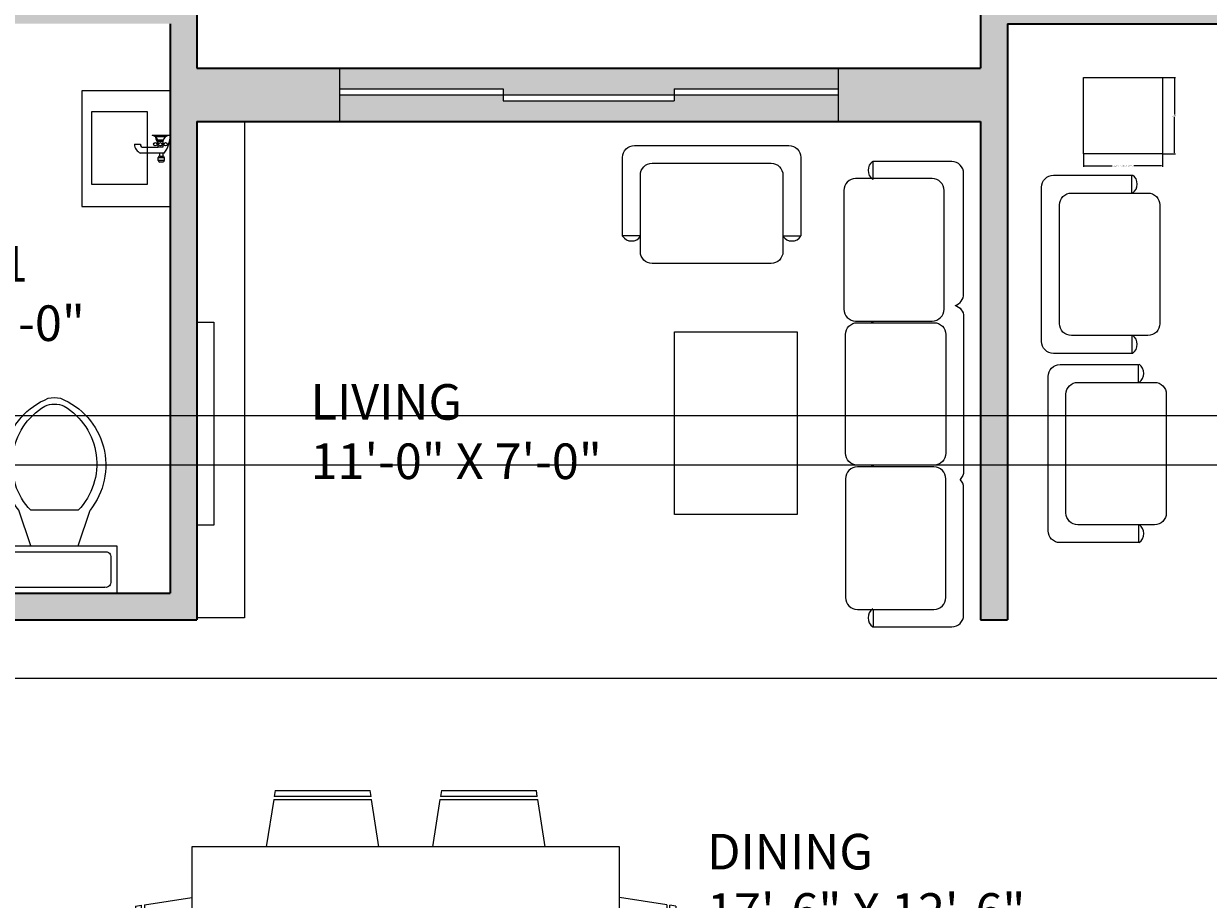
# Model space of a CAD drawing. Units: inches. Extents: x 1693 to 2974, y 2201 to 2965.
# Tile 12 of 24: x 1976 to 2175, y 2550 to 2698. Entities that reach past the tile are written whole.
import ezdxf

# ---------------------------------------------------------------- set-up
doc = ezdxf.new("R2010")
doc.units = ezdxf.units.IN
doc.header["$LTSCALE"] = 2
doc.header["$MEASUREMENT"] = 0
for name, color, linetype, lineweight in [('A-ANNO-DIMS', 2, 'Continuous', 18), ('A-AREA-IDEN', 7, 'Continuous', 18), ('A-DOOR', 3, 'Continuous', 25), ('A-FLOR-FIXT', 9, 'Continuous', 18), ('A-FURN', 8, 'Continuous', 18), ('A-WALL', 7, 'Continuous', 35)]:
    doc.layers.add(name, color=color, linetype=linetype, lineweight=lineweight)
doc.layers.add('A-GLAZ-PATT', color=141, linetype='Continuous', lineweight=13, true_color=0xadddf7)
doc.layers.add('A-WALL-PATT', color=251, linetype='Continuous', lineweight=13, true_color=0x636466)
doc.styles.get("Standard").update_dxf_attribs({"font": 'arial.ttf'})
doc.dimstyles.get("Standard").update_dxf_attribs({"dimtxt": 0.18, "dimasz": 0.18, "dimexe": 0.18, "dimexo": 0.0625, "dimgap": 0.09, "dimtad": 0, "dimtih": 1, "dimtoh": 1, "dimdec": 1, "dimzin": 0, "dimdsep": 46, "dimlunit": 3, "dimtxsty": 'Standard', "dimcen": 0.09, "dimadec": 0, "dimazin": 0, "dimtfac": 1, "dimtdec": 1, "dimtofl": 0, "dimtmove": 0, "dimatfit": 3, "dimfxl": 1, "dimtolj": 1, "dimtzin": 0, "dimarcsym": 0})

# ---------------------------------------------------------------- blocks, each defined once
blk = doc.blocks.new('Faucet - Bathroom side')
for p, q in [((-0.625, 4.25), (0.375, 4.25)), ((0.375, 3.75), (-0.625, 3.75)), ((-0.625, 3), (3.375, 3)), ((-0.375, 3), (-0.375, 3.5)), ((0.125, 3.5), (0.125, 3)), ((2.875, 2), (0.375, 2)), ((-1.625, 0), (-1.375, 0)), ((-1.375, 0), (1.375, 0)), ((-0.88366, 0.25), (0.88424, 0.25)), ((-0.375, 1.625), (-0.625, 1.625)), ((-0.375, 1.375), (-0.625, 1.375)), ((0.48078, 0.75), (-0.47286, 0.75)), ((0.375, 1.625), (0.625, 1.625)), ((0.375, 1.375), (0.625, 1.375)), ((4.375, 1.5), (3.375, 1.5))]:
    blk.add_line(p, q)
for points in [[(-0.625, 3.75), (-0.625, 4.25)], [(-0.375, 4.5), (0.125, 4.5)], [(0.375, 4.25), (0.375, 3.75)], [(0.125, 3.5), (-0.375, 3.5)]]:
    blk.add_lwpolyline(points)
blk.add_lwpolyline([(-0.375, 1), (-0.375, 2), (0.375, 2), (0.375, 1)], close=True)
for centre in [(-0.875, 1.5), (0, 1.5), (0.875, 1.5)]:
    blk.add_circle(centre, 0.27951)
for centre, radius, start, end in [((-0.38253, 4.2575), 0.24259, 88.22243, 181.7776), ((0.13252, 4.2575), 0.24259, 358.2224, 91.77757), ((3.45929, -0.0281), 5.08436, 143.4467, 179.6834), ((-0.38253, 3.7424), 0.24259, 178.2224, 271.7776), ((0.13252, 3.7424), 0.24259, 268.2224, 1.777565), ((2.96867, 1.5936), 0.41699, 347.0192, 102.9808), ((2.70708, 1.4714), 1.66816, 0.9827695, 66.39737), ((-1.75, 1.375), 1.42522, 285.2551, 344.7449), ((1.75, 1.375), 1.42522, 195.2551, 254.7449), ((-2.49562, -0.286), 3.38273, 9.709485, 29.48735)]:
    blk.add_arc(centre, radius, start, end)
blk = doc.blocks.new('Toilet - top')
for p, q in [((9.5, -6), (9.5, -2)), ((-10, -8.5), (-8, -8.5)), ((-10, -9.5), (-10, -8.5)), ((-7, -9.5), (-10, -9.5)), ((-8, -8.5), (-8, -8)), ((-7, -8), (-7, -9.5)), ((-4, -8), (-6, -14)), ((4, -8), (6, -14)), ((4, -14), (-4, -14))]:
    blk.add_line(p, q)
blk.add_lwpolyline([(10.5, -8), (10.5, 0), (-10.5, 0), (-10.5, -8)], close=True)
for points in [[(8.5, -1), (-8.5, -1)], [(-9.5, -2), (-9.5, -6)], [(-8.5, -7), (8.5, -7)]]:
    blk.add_lwpolyline(points)
for centre, radius, start, end in [((-8.62, -1.88), 0.884, 81.8699, 188.1301), ((8.62, -1.88), 0.884, 351.8699, 98.1301), ((-8.62, -6.12), 0.884, 171.8699, 278.1301), ((8.62, -6.12), 0.884, 261.8699, 8.1301), ((3.52, -21.58), 12.17, 141.4691, 247.9714), ((4.2, -21.82), 11.33, 136.3677, 238.9468), ((-3.52, -21.58), 12.17, 292.0284, 38.5307), ((-4.2, -21.82), 11.33, 301.053, 43.6321), ((0, -27.88), 4, 245.7318, 294.2682), ((0, -29), 4, 254.8605, 285.1395)]:
    blk.add_arc(centre, radius, start, end)
blk = doc.blocks.new('DINING-SET-72x36-6-SEAT')
for p, q in [((23.5, 55), (23.34, 54)), ((39.66, 54), (23.35, 54)), ((23.5, 55), (39.5, 55)), ((39.66, 54), (39.5, 55)), ((51.5, 55), (51.34, 54)), ((67.66, 54), (51.35, 54)), ((51.5, 55), (67.5, 55)), ((67.66, 54), (67.5, 55)), ((23.27, 53.5), (22.02, 45.5)), ((23.27, 53.5), (39.74, 53.5)), ((40.98, 45.5), (39.73, 53.5)), ((51.27, 53.5), (50.02, 45.5)), ((51.27, 53.5), (67.74, 53.5)), ((68.98, 45.5), (67.73, 53.5)), ((81.5, 45.5), (9.5, 45.5)), ((9.5, 45.5), (9.5, 9.5)), ((81.5, 9.5), (81.5, 45.5)), ((1.5, 35.73), (9.5, 36.98)), ((89.5, 35.73), (81.5, 36.98)), ((0, 35.5), (1, 35.66)), ((0, 35.5), (0, 19.5)), ((1, 19.34), (1, 35.65)), ((1.5, 35.73), (1.5, 19.26)), ((89.5, 35.73), (89.5, 19.26)), ((91, 35.5), (90, 35.66)), ((90, 19.34), (90, 35.65)), ((91, 35.5), (91, 19.5)), ((1, 19.34), (0, 19.5)), ((9.5, 18.02), (1.5, 19.27)), ((81.5, 18.02), (89.5, 19.27)), ((90, 19.34), (91, 19.5)), ((9.5, 9.5), (81.5, 9.5)), ((23.27, 1.5), (22.02, 9.5)), ((40.98, 9.5), (39.73, 1.5)), ((51.27, 1.5), (50.02, 9.5)), ((68.98, 9.5), (67.73, 1.5)), ((23.27, 1.5), (39.74, 1.5)), ((23.5, 0), (23.34, 1)), ((39.66, 1), (23.35, 1)), ((23.5, 0), (39.5, 0)), ((39.66, 1), (39.5, 0)), ((51.27, 1.5), (67.74, 1.5)), ((51.5, 0), (51.34, 1)), ((67.66, 1), (51.35, 1)), ((51.5, 0), (67.5, 0)), ((67.66, 1), (67.5, 0))]:
    blk.add_line(p, q)
blk = doc.blocks.new('LOUNGE-CHAIR-A')
at = {"ltscale": 2}
for p, q in [((15.21, 27.01), (15.21, 30.01)), ((15.21, 3), (15.21, 0))]:
    blk.add_line(p, q, dxfattribs=at)
for points in [[(15.31, 0), (2, 0, -0.414214), (0, 2), (0, 28.01, -0.414214), (2, 30.01), (15.21, 30.01)], [(19.9, 5, -0.414214), (17.9, 3), (5, 3, -0.414214), (3, 5), (3, 25.01, -0.414214), (5, 27.01), (17.9, 27.01, -0.414214), (19.9, 25.01), (19.9, 5)]]:
    blk.add_lwpolyline(points, format="xyb", dxfattribs=at)
for centre in [(14.24, 28.53), (14.24, 1.52)]:
    blk.add_arc(centre, 1.86, 305.0084, 54.9916, dxfattribs=at)
blk = doc.blocks.new('TABLE-END-SQUARE')
at = {"ltscale": 2}
blk.add_lwpolyline([(0, 12.88), (13.32, 12.88), (13.32, 0), (0, 0)], close=True, dxfattribs=at)
blk = doc.blocks.new('*D71')
at = {"layer": 'A-ANNO-DIMS', "color": 0, "lineweight": -2, "ltscale": 2, "transparency": 16777216}
for p, q in [((2154.05, 2675.84), (2154.05, 2673.72)), ((2167.37, 2675.84), (2167.37, 2673.72)), ((2154.23, 2673.9), (2158.89, 2673.9)), ((2167.19, 2673.9), (2162.54, 2673.9))]:
    blk.add_line(p, q, dxfattribs=at)
at = {"layer": 'A-ANNO-DIMS', "color": 0, "ltscale": 2, "transparency": 16777216}
for points in [[(2154.23, 2673.93), (2154.23, 2673.87), (2154.05, 2673.9)], [(2167.19, 2673.93), (2167.19, 2673.87), (2167.37, 2673.9)]]:
    blk.add_solid(points, dxfattribs=at)
at = {"layer": 'Defpoints', "color": 0, "ltscale": 2, "transparency": 16777216}
for p in [(2154.05, 2675.9), (2167.37, 2675.9), (2167.37, 2673.9)]:
    blk.add_point(p, dxfattribs=at)
at = {"layer": 'A-ANNO-DIMS', "color": 0, "ltscale": 2, "transparency": 16777216, "insert": (2160.71, 2673.9), "char_height": 0.18, "attachment_point": 5}
blk.add_mtext('\\A1;SQUARE END TABLE 13 TYP.', dxfattribs=at)
blk = doc.blocks.new('*D72')
at = {"layer": 'A-ANNO-DIMS', "color": 0, "lineweight": -2, "ltscale": 2, "transparency": 16777216}
for p, q in [((2167.44, 2688.78), (2169.55, 2688.78)), ((2169.37, 2688.6), (2169.37, 2682.52)), ((2169.37, 2676.08), (2169.37, 2682.16)), ((2167.44, 2675.9), (2169.55, 2675.9))]:
    blk.add_line(p, q, dxfattribs=at)
at = {"layer": 'A-ANNO-DIMS', "color": 0, "ltscale": 2, "transparency": 16777216}
for points in [[(2169.34, 2688.6), (2169.4, 2688.6), (2169.37, 2688.78)], [(2169.34, 2676.08), (2169.4, 2676.08), (2169.37, 2675.9)]]:
    blk.add_solid(points, dxfattribs=at)
at = {"layer": 'Defpoints', "color": 0, "ltscale": 2, "transparency": 16777216}
for p in [(2167.37, 2688.78), (2169.37, 2688.78), (2167.37, 2675.9)]:
    blk.add_point(p, dxfattribs=at)
at = {"layer": 'A-ANNO-DIMS', "color": 0, "ltscale": 2, "transparency": 16777216, "insert": (2169.37, 2682.34), "char_height": 0.18, "attachment_point": 5}
blk.add_mtext('\\A1;13 TYP.', dxfattribs=at)
blk = doc.blocks.new('*D81')
at = {"layer": 'A-ANNO-DIMS', "color": 0, "lineweight": -2, "ltscale": 2, "transparency": 16777216}
for p, q in [((1752.34, 2553.91), (1752.34, 2964.96)), ((1752.52, 2964.78), (2332.94, 2964.78)), ((2914.06, 2964.78), (2333.64, 2964.78)), ((2914.24, 2754.97), (2914.24, 2964.96))]:
    blk.add_line(p, q, dxfattribs=at)
at = {"layer": 'A-ANNO-DIMS', "color": 0, "ltscale": 2, "transparency": 16777216}
for points in [[(1752.52, 2964.81), (1752.52, 2964.75), (1752.34, 2964.78)], [(2914.06, 2964.81), (2914.06, 2964.75), (2914.24, 2964.78)]]:
    blk.add_solid(points, dxfattribs=at)
at = {"layer": 'Defpoints', "color": 0, "ltscale": 2, "transparency": 16777216}
for p in [(2914.24, 2964.78), (2914.24, 2754.9), (1752.34, 2553.84)]:
    blk.add_point(p, dxfattribs=at)
at = {"layer": 'A-ANNO-DIMS', "color": 0, "ltscale": 2, "transparency": 16777216, "insert": (2333.29, 2964.78), "char_height": 0.18, "attachment_point": 5}
blk.add_mtext('\\A1;1162', dxfattribs=at)
blk = doc.blocks.new('*D82')
at = {"layer": 'A-ANNO-DIMS', "color": 0, "lineweight": -2, "ltscale": 2, "transparency": 16777216}
for p, q in [((2615.67, 2906.08), (1693.46, 2906.08)), ((1693.64, 2905.9), (1693.64, 2582.94)), ((1693.64, 2259.62), (1693.64, 2582.58)), ((2096.17, 2259.44), (1693.46, 2259.44))]:
    blk.add_line(p, q, dxfattribs=at)
at = {"layer": 'A-ANNO-DIMS', "color": 0, "ltscale": 2, "transparency": 16777216}
for points in [[(1693.61, 2905.9), (1693.67, 2905.9), (1693.64, 2906.08)], [(1693.61, 2259.62), (1693.67, 2259.62), (1693.64, 2259.44)]]:
    blk.add_solid(points, dxfattribs=at)
at = {"layer": 'Defpoints', "color": 0, "ltscale": 2, "transparency": 16777216}
for p in [(1693.64, 2906.08), (2615.74, 2906.08), (2096.24, 2259.44)]:
    blk.add_point(p, dxfattribs=at)
at = {"layer": 'A-ANNO-DIMS', "color": 0, "ltscale": 2, "transparency": 16777216, "insert": (1693.64, 2582.76), "char_height": 0.18, "attachment_point": 5}
blk.add_mtext('\\A1;646.6', dxfattribs=at)
blk = doc.blocks.new('*D88')
at = {"layer": 'A-ANNO-DIMS', "color": 0, "lineweight": -2, "ltscale": 2, "transparency": 16777216}
for p, q in [((2479.17, 2700.75), (1693.46, 2700.75)), ((1693.64, 2700.57), (1693.64, 2666.44)), ((1693.64, 2631.93), (1693.64, 2666.07)), ((2479.17, 2631.75), (1693.46, 2631.75))]:
    blk.add_line(p, q, dxfattribs=at)
at = {"layer": 'A-ANNO-DIMS', "color": 0, "ltscale": 2, "transparency": 16777216}
for points in [[(1693.61, 2700.57), (1693.67, 2700.57), (1693.64, 2700.75)], [(1693.61, 2631.93), (1693.67, 2631.93), (1693.64, 2631.75)]]:
    blk.add_solid(points, dxfattribs=at)
at = {"layer": 'Defpoints', "color": 0, "ltscale": 2, "transparency": 16777216}
for p in [(1693.64, 2700.75), (2479.24, 2700.75), (2479.24, 2631.75)]:
    blk.add_point(p, dxfattribs=at)
at = {"layer": 'A-ANNO-DIMS', "color": 0, "ltscale": 2, "transparency": 16777216, "insert": (1693.64, 2666.25), "char_height": 0.18, "attachment_point": 5}
blk.add_mtext('\\A1;69', dxfattribs=at)
blk = doc.blocks.new('*D98')
at = {"layer": 'A-ANNO-DIMS', "color": 0, "lineweight": -2, "ltscale": 2, "transparency": 16777216}
for p, q in [((2479.17, 2623.46), (1693.46, 2623.46)), ((1693.64, 2623.28), (1693.64, 2605.64)), ((1693.64, 2587.64), (1693.64, 2605.28)), ((2479.17, 2587.46), (1693.46, 2587.46))]:
    blk.add_line(p, q, dxfattribs=at)
at = {"layer": 'A-ANNO-DIMS', "color": 0, "ltscale": 2, "transparency": 16777216}
for points in [[(1693.61, 2623.28), (1693.67, 2623.28), (1693.64, 2623.46)], [(1693.61, 2587.64), (1693.67, 2587.64), (1693.64, 2587.46)]]:
    blk.add_solid(points, dxfattribs=at)
at = {"layer": 'Defpoints', "color": 0, "ltscale": 2, "transparency": 16777216}
for p in [(1693.64, 2623.46), (2479.24, 2623.46), (2479.24, 2587.46)]:
    blk.add_point(p, dxfattribs=at)
at = {"layer": 'A-ANNO-DIMS', "color": 0, "ltscale": 2, "transparency": 16777216, "insert": (1693.64, 2605.46), "char_height": 0.18, "attachment_point": 5}
blk.add_mtext('\\A1;36', dxfattribs=at)
blk = doc.blocks.new('*D99')
at = {"layer": 'A-ANNO-DIMS', "color": 0, "lineweight": -2, "ltscale": 2, "transparency": 16777216}
for p, q in [((2479.17, 2631.75), (1693.46, 2631.75)), ((1693.64, 2631.57), (1693.64, 2627.79)), ((1693.64, 2623.64), (1693.64, 2627.43)), ((2479.17, 2623.46), (1693.46, 2623.46))]:
    blk.add_line(p, q, dxfattribs=at)
at = {"layer": 'A-ANNO-DIMS', "color": 0, "ltscale": 2, "transparency": 16777216}
for points in [[(1693.61, 2631.57), (1693.67, 2631.57), (1693.64, 2631.75)], [(1693.61, 2623.64), (1693.67, 2623.64), (1693.64, 2623.46)]]:
    blk.add_solid(points, dxfattribs=at)
at = {"layer": 'Defpoints', "color": 0, "ltscale": 2, "transparency": 16777216}
for p in [(1693.64, 2631.75), (2479.24, 2631.75), (2479.24, 2623.46)]:
    blk.add_point(p, dxfattribs=at)
at = {"layer": 'A-ANNO-DIMS', "color": 0, "ltscale": 2, "transparency": 16777216, "insert": (1693.64, 2627.61), "char_height": 0.18, "attachment_point": 5}
blk.add_mtext('\\A1;8.295', dxfattribs=at)

msp = doc.modelspace()

# ---------------------------------------------------------------- hatches: boundary and pattern name
at = {"layer": 'A-GLAZ-PATT', "ltscale": 2}
h = msp.add_hatch(color=256, dxfattribs=at)
h.dxf.hatch_style = 1
h.paths.add_polyline_path([(2656.9702, 2338.2547), (2632.9702, 2338.2547), (2632.9702, 2339.2547), (2608.9702, 2339.2547), (2608.9702, 2334.7547), (2656.9702, 2334.7547)])
h.paths.add_polyline_path([(2656.9702, 2343.7547), (2608.9702, 2343.7547), (2608.9702, 2340.2547), (2632.9702, 2340.2547), (2632.9702, 2339.2547), (2656.9702, 2339.2547)])
h.paths.add_polyline_path([(2775.7544, 2338.2547), (2751.7544, 2338.2547), (2751.7544, 2334.7547), (2775.7544, 2334.7547)])
h.paths.add_polyline_path([(2775.7544, 2343.7547), (2751.7544, 2343.7547), (2751.7544, 2340.2547), (2775.7544, 2340.2547)])
h.paths.add_polyline_path([(2897.7363, 2568.7999), (2893.2363, 2568.7999), (2893.2363, 2520.7999), (2896.7363, 2520.7999), (2896.7363, 2544.7999), (2897.7363, 2544.7999)])
h.paths.add_polyline_path([(2902.2363, 2568.7999), (2898.7363, 2568.7999), (2898.7363, 2544.7999), (2897.7363, 2544.7999), (2897.7363, 2520.7999), (2902.2363, 2520.7999)])
h.paths.add_polyline_path([(2902.2363, 2637.7547), (2898.7363, 2637.7547), (2898.7363, 2613.7547), (2902.2363, 2613.7547)])
h.paths.add_polyline_path([(2896.7363, 2637.7547), (2893.2363, 2637.7547), (2893.2363, 2613.7547), (2896.7363, 2613.7547)])
h.paths.add_polyline_path([(2902.2363, 2748.903), (2899.0477, 2748.903), (2899.0477, 2724.903), (2898.0477, 2724.903), (2898.0477, 2700.903), (2902.2363, 2700.903)])
h.paths.add_polyline_path([(2898.0477, 2748.903), (2893.2363, 2748.903), (2893.2363, 2700.903), (2897.0477, 2700.903), (2897.0477, 2724.903), (2898.0477, 2724.903)])
h.paths.add_polyline_path([(2851.2363, 2846.2547), (2803.2363, 2846.2547), (2803.2363, 2842.7547), (2827.2363, 2842.7547), (2827.2363, 2841.7547), (2851.2363, 2841.7547)])
h.paths.add_polyline_path([(2851.2363, 2840.7547), (2827.2363, 2840.7547), (2827.2363, 2841.7547), (2803.2363, 2841.7547), (2803.2363, 2837.2547), (2851.2363, 2837.2547)])
h.paths.add_polyline_path([(2578.2363, 2846.2547), (2530.2363, 2846.2547), (2530.2363, 2842.7547), (2554.2363, 2842.7547), (2554.2363, 2841.7547), (2578.2363, 2841.7547)])
h.paths.add_polyline_path([(2578.2363, 2840.7547), (2554.2363, 2840.7547), (2554.2363, 2841.7547), (2530.2363, 2841.7547), (2530.2363, 2837.2547), (2578.2363, 2837.2547)])
h.paths.add_polyline_path([(2732.7363, 2812.7547), (2705.1363, 2812.7547), (2705.1363, 2811.7547), (2676.3363, 2811.7547), (2676.3363, 2812.7547), (2648.7363, 2812.7547), (2648.7363, 2808.2547), (2732.7363, 2808.2547)])
h.paths.add_polyline_path([(2732.7363, 2817.2547), (2648.7363, 2817.2547), (2648.7363, 2813.7547), (2676.3363, 2813.7547), (2676.3363, 2812.7547), (2705.1363, 2812.7547), (2705.1363, 2813.7547), (2732.7363, 2813.7547)])
h.paths.add_polyline_path([(2488.2363, 2695.8203), (2484.7878, 2695.8203), (2484.7878, 2671.8203), (2488.2363, 2671.8203)])
h.paths.add_polyline_path([(2482.7878, 2695.8203), (2479.2363, 2695.8203), (2479.2363, 2671.8203), (2482.7878, 2671.8203)])
h.paths.add_polyline_path([(2488.2363, 2572.4371), (2484.7363, 2572.4371), (2484.7363, 2541.4371), (2483.7363, 2541.4371), (2483.7363, 2512.4371), (2488.2363, 2512.4371)])
h.paths.add_polyline_path([(2482.7363, 2541.4371), (2483.7363, 2541.4371), (2483.7363, 2572.4371), (2479.2363, 2572.4371), (2479.2363, 2512.4371), (2482.7363, 2512.4371)])
h.paths.add_polyline_path([(2248.9863, 2706.8449), (2190.9863, 2706.8449), (2190.9863, 2703.3449), (2219.9863, 2703.3449), (2219.9863, 2702.3449), (2248.9863, 2702.3449)])
h.paths.add_polyline_path([(2248.9863, 2701.3449), (2219.9863, 2701.3449), (2219.9863, 2702.3449), (2190.9863, 2702.3449), (2190.9863, 2697.8449), (2248.9863, 2697.8449)])
h.paths.add_polyline_path([(2151.9207, 2293.3449), (2127.9207, 2293.3449), (2127.9207, 2289.8449), (2151.9207, 2289.8449)])
h.paths.add_polyline_path([(2151.9207, 2298.8449), (2127.9207, 2298.8449), (2127.9207, 2295.3449), (2151.9207, 2295.3449)])
h.paths.add_polyline_path([(2084.023, 2293.3449), (2066.023, 2293.3449), (2066.023, 2294.3449), (2048.023, 2294.3449), (2048.023, 2289.8449), (2084.023, 2289.8449)])
h.paths.add_polyline_path([(2084.023, 2298.8449), (2048.023, 2298.8449), (2048.023, 2295.3449), (2066.023, 2295.3449), (2066.023, 2294.3449), (2084.023, 2294.3449)])
h.paths.add_polyline_path([(1966.0781, 2293.3449), (1948.0781, 2293.3449), (1948.0781, 2294.3449), (1930.0781, 2294.3449), (1930.0781, 2289.8449), (1966.0781, 2289.8449)])
h.paths.add_polyline_path([(1966.0781, 2298.8449), (1930.0781, 2298.8449), (1930.0781, 2295.3449), (1948.0781, 2295.3449), (1948.0781, 2294.3449), (1966.0781, 2294.3449)])
h.paths.add_polyline_path([(1787.2363, 2403.1922), (1782.7363, 2403.1922), (1782.7363, 2355.1922), (1786.2363, 2355.1922), (1786.2363, 2379.1922), (1787.2363, 2379.1922)])
h.paths.add_polyline_path([(1791.7363, 2403.1922), (1788.2363, 2403.1922), (1788.2363, 2379.1922), (1787.2363, 2379.1922), (1787.2363, 2355.1922), (1791.7363, 2355.1922)])
h.paths.add_polyline_path([(1786.2363, 2477.5455), (1782.7363, 2477.5455), (1782.7363, 2453.5455), (1786.2363, 2453.5455)])
h.paths.add_polyline_path([(1791.7363, 2477.5455), (1788.2363, 2477.5455), (1788.2363, 2453.5455), (1791.7363, 2453.5455)])
h.paths.add_polyline_path([(1786.2363, 2621.6433), (1782.7363, 2621.6433), (1782.7363, 2585.6433), (1786.2363, 2585.6433)])
h.paths.add_polyline_path([(1791.7363, 2621.6433), (1788.2363, 2621.6433), (1788.2363, 2585.6433), (1791.7363, 2585.6433)])
h.paths.add_polyline_path([(1908.1286, 2706.8449), (1860.1286, 2706.8449), (1860.1286, 2703.3449), (1884.1286, 2703.3449), (1884.1286, 2702.3449), (1908.1286, 2702.3449)])
h.paths.add_polyline_path([(1908.1286, 2701.3449), (1884.1286, 2701.3449), (1884.1286, 2702.3449), (1860.1286, 2702.3449), (1860.1286, 2697.8449), (1908.1286, 2697.8449)])
h.paths.add_polyline_path([(1973.9863, 2706.8449), (1949.9863, 2706.8449), (1949.9863, 2703.3449), (1973.9863, 2703.3449)])
h.paths.add_polyline_path([(1973.9863, 2701.3449), (1949.9863, 2701.3449), (1949.9863, 2697.8449), (1973.9863, 2697.8449)])
h.paths.add_polyline_path([(2112.7363, 2690.3449), (2028.7363, 2690.3449), (2028.7363, 2686.8449), (2056.3363, 2686.8449), (2056.3363, 2685.8449), (2085.1363, 2685.8449), (2085.1363, 2686.8449), (2112.7363, 2686.8449)])
h.paths.add_polyline_path([(2112.7363, 2685.8449), (2085.1363, 2685.8449), (2085.1363, 2684.8449), (2056.3363, 2684.8449), (2056.3363, 2685.8449), (2028.7363, 2685.8449), (2028.7363, 2681.3449), (2112.7363, 2681.3449)])
h.paths.add_polyline_path([(2422.7363, 2640.7547), (2350.7363, 2640.7547), (2350.7363, 2637.2547), (2386.7363, 2637.2547), (2386.7363, 2636.2547), (2422.7363, 2636.2547)])
h.paths.add_polyline_path([(2422.7363, 2635.2547), (2386.7363, 2635.2547), (2386.7363, 2636.2547), (2350.7363, 2636.2547), (2350.7363, 2631.7547), (2422.7363, 2631.7547)])
at = {"layer": 'A-WALL-PATT', "ltscale": 2}
h = msp.add_hatch(color=256, dxfattribs=at)
h.dxf.hatch_style = 1
h.paths.add_polyline_path([(1928.2363, 2733.2161), (1930.9384, 2733.2161), (1930.9384, 2737.2161), (1923.7363, 2737.2161), (1923.7363, 2706.8449), (1908.1286, 2706.8449), (1908.1286, 2697.8449), (1923.7363, 2697.8449), (1923.7363, 2692.8449), (1928.2363, 2692.8449), (1928.2363, 2697.8449), (1949.9863, 2697.8449), (1949.9863, 2706.8449), (1928.2363, 2706.8449)])
h.paths.add_polyline_path([(2004.7363, 2737.2161), (1995.7363, 2737.2161), (1995.7363, 2706.8449), (1985.6374, 2706.8449), (1973.9863, 2706.8449), (1973.9863, 2697.8449), (2000.2363, 2697.8449), (2000.2363, 2686.5348), (2000.3613, 2686.5348), (2000.3613, 2667.0432), (2000.2363, 2601.8449), (1928.2363, 2601.8449), (1928.2363, 2662.8449), (1923.7363, 2662.8449), (1923.7363, 2595.3449), (1928.2363, 2595.3449), (1928.2363, 2597.3449), (2004.7363, 2597.3449), (2004.7363, 2681.3449), (2012.7814, 2681.3449), (2028.7363, 2681.3449), (2028.7363, 2690.3449), (2004.7363, 2690.3449)])
h.paths.add_polyline_path([(2190.9863, 2706.8449), (2184.9863, 2706.8449), (2145.7363, 2706.8449), (2145.7363, 2765.3449), (2145.7363, 2774.5394), (2136.7363, 2774.5394), (2136.7363, 2756.3449), (2136.7363, 2690.3449), (2112.7363, 2690.3449), (2112.7363, 2681.3449), (2136.7363, 2681.3449), (2136.7363, 2597.3449), (2141.2363, 2597.3449), (2141.2363, 2697.8449), (2190.9863, 2697.8449)])
h.paths.add_polyline_path([(1860.1286, 2706.8449), (1782.7363, 2706.8449), (1782.7363, 2621.6433), (1791.7363, 2621.6433), (1791.7363, 2697.8449), (1860.1286, 2697.8449)])
h.paths.add_polyline_path([(1791.7363, 2585.6433), (1782.7363, 2585.6433), (1782.7363, 2562.8449), (1782.7363, 2553.8449), (1752.3363, 2553.8449), (1752.3363, 2544.2586), (1756.3363, 2544.2586), (1756.3363, 2549.3449), (1782.7363, 2549.3449), (1782.7363, 2489.2404), (1782.7363, 2477.5455), (1791.7363, 2477.5455), (1791.7363, 2493.5991), (1791.6113, 2493.5991), (1791.6113, 2513.0907), (1791.6824, 2533.7198, -0.94742783), (1791.7363, 2534.7168), (1791.7363, 2549.3449), (1863.7363, 2549.3449), (1863.7363, 2513.3449), (1866.7363, 2513.3449), (1866.7363, 2549.3449), (1924.7363, 2549.3449), (1924.7363, 2447.3449), (1924.7363, 2442.8449), (1933.7363, 2442.8449), (1933.7363, 2447.3449), (1928.2363, 2447.3449), (1928.2363, 2559.3449), (1923.7363, 2559.3449), (1923.7363, 2553.8449), (1791.7363, 2553.8449), (1791.7363, 2562.8449)])
h.paths.add_polyline_path([(1791.7363, 2442.8449), (1866.7363, 2442.8449), (1866.7363, 2447.3449), (1866.7363, 2483.3449), (1863.7363, 2483.3449), (1863.7363, 2447.3449), (1791.7363, 2447.3449), (1791.7363, 2453.5455), (1782.7363, 2453.5455), (1782.7363, 2447.3449), (1756.3363, 2447.3449), (1756.3363, 2455.7126), (1752.3363, 2455.7126), (1752.3363, 2442.8449), (1782.7363, 2442.8449), (1782.7363, 2403.1922), (1791.7363, 2403.1922)])
h.paths.add_polyline_path([(1930.0781, 2298.8449), (1791.7363, 2298.8449), (1791.7363, 2355.1922), (1782.7363, 2355.1922), (1782.7363, 2289.8449), (1930.0781, 2289.8449)])
h.paths.add_polyline_path([(2624.7363, 2883.2547), (2624.7363, 2902.6165), (2624.7363, 2906.0761), (2615.7363, 2906.0761), (2615.7363, 2892.2547), (2615.7363, 2846.2547), (2578.2363, 2846.2547), (2578.2363, 2837.2547), (2620.2363, 2837.2547), (2620.2363, 2743.2547), (2624.7363, 2743.2547), (2624.7363, 2808.2547), (2648.7363, 2808.2547), (2648.7363, 2817.2547), (2624.7363, 2817.2547)])
h.paths.add_polyline_path([(2530.2363, 2846.2547), (2479.2363, 2846.2547), (2479.2363, 2695.8203), (2488.2363, 2695.8203), (2488.2363, 2700.7547), (2567.2363, 2700.7547), (2567.2363, 2705.2547), (2488.2363, 2705.2547), (2488.2363, 2837.2547), (2530.2363, 2837.2547)])
h.paths.add_polyline_path([(2488.2363, 2487.7547), (2630.2363, 2487.7547, -0.00990191), (2630.2363, 2489.0322), (2630.2363, 2492.2547), (2488.2363, 2492.2547), (2488.2363, 2512.4371), (2479.2363, 2512.4371), (2479.2363, 2334.7547), (2608.9702, 2334.7547), (2608.9702, 2343.7547), (2488.2363, 2343.7547)])
h.paths.add_polyline_path([(2751.7544, 2343.7547), (2672.7363, 2343.7547), (2672.7363, 2409.7547), (2674.7363, 2409.7547), (2674.7363, 2413.7547), (2672.7363, 2413.7547), (2672.7363, 2487.7547), (2732.7363, 2487.7547), (2732.7363, 2413.7547), (2704.7363, 2413.7547), (2704.7363, 2409.7547), (2784.7363, 2409.7547), (2784.7363, 2343.7547), (2775.7544, 2343.7547), (2775.7544, 2334.7547), (2902.2363, 2334.7547), (2902.2363, 2520.7999), (2893.2363, 2520.7999), (2893.2363, 2413.7547), (2856.0145, 2413.7547), (2856.0145, 2409.7547), (2893.2363, 2409.7547), (2893.2363, 2343.7547), (2789.2363, 2343.7547), (2789.2363, 2409.7547), (2819.2363, 2409.7547), (2826.0145, 2409.7547), (2826.0145, 2413.7547), (2789.2363, 2413.7547), (2789.2363, 2492.2547), (2784.7363, 2492.2547), (2784.7363, 2413.7547), (2736.7363, 2413.7547), (2736.7363, 2492.2547), (2672.7363, 2492.2547), (2666.2363, 2492.2547), (2666.2363, 2487.7547), (2668.2363, 2487.7547), (2668.2363, 2343.7547), (2656.9702, 2343.7547), (2656.9702, 2334.7547), (2662.9702, 2334.7547), (2751.7544, 2334.7547)])
h.paths.add_polyline_path([(2902.2363, 2613.7547), (2893.2363, 2613.7547), (2893.2363, 2589.7547), (2785.2363, 2589.7547), (2785.2363, 2661.7547), (2790.2363, 2661.7547), (2790.2363, 2665.2547), (2761.2363, 2665.2547), (2761.2363, 2667.2547), (2756.7363, 2667.2547), (2756.7363, 2661.7547), (2781.2363, 2661.7547), (2781.2363, 2585.7547), (2893.2363, 2585.7547), (2893.2363, 2568.7999), (2902.2363, 2568.7999)])
h.paths.add_polyline_path([(2488.2363, 2671.8203), (2479.2363, 2671.8203), (2479.2363, 2645.2547), (2479.2363, 2623.4598), (2488.2363, 2623.4598), (2488.2363, 2636.2547), (2624.7363, 2636.2547), (2624.7363, 2640.7547), (2603.7363, 2640.7547), (2603.7363, 2700.7547), (2624.7363, 2700.7547), (2624.7363, 2707.2547), (2620.2363, 2707.2547), (2620.2363, 2705.2547), (2597.2363, 2705.2547), (2597.2363, 2700.7547), (2599.2363, 2700.7547), (2599.2363, 2640.7547), (2488.2363, 2640.7547)])
h.paths.add_polyline_path([(2761.2363, 2837.2547), (2803.2363, 2837.2547), (2803.2363, 2846.2547), (2797.2363, 2846.2547), (2765.7363, 2846.2547), (2756.7363, 2846.2547), (2756.7363, 2817.2547), (2732.7363, 2817.2547), (2732.7363, 2808.2547), (2756.7363, 2808.2547), (2756.7363, 2703.2547), (2761.2363, 2703.2547)])
h.paths.add_polyline_path([(2739.7489, 2433.1234), (2786.9181, 2433.1234), (2786.9181, 2455.5122), (2739.7489, 2455.5122)], flags=25)

# ---------------------------------------------------------------- linework, layer by layer
at = {"layer": 'A-DOOR', "ltscale": 2}
for p, q in [((2028.7363, 2690.3449), (2028.7363, 2681.3449)), ((2112.7363, 2690.3449), (2112.7363, 2681.3449)), ((2028.7363, 2686.8449), (2056.3363, 2686.8449)), ((2028.7363, 2685.8449), (2112.7363, 2685.8449)), ((2056.3363, 2686.8449), (2056.3363, 2684.8449)), ((2085.1363, 2686.8449), (2085.1363, 2684.8449)), ((2085.1363, 2686.8449), (2112.7363, 2686.8449)), ((2056.3363, 2684.8449), (2085.1363, 2684.8449))]:
    msp.add_line(p, q, dxfattribs=at)
at = {"layer": 'A-FLOR-FIXT', "ltscale": 2}
for points in [[(2000.3613, 2686.5348), (1985.3475, 2686.5348), (1985.3475, 2667.0432), (2000.3613, 2667.0432)], [(1996.4485, 2682.9811), (1986.9793, 2682.9811), (1986.9793, 2670.7988), (1996.4485, 2670.7988)]]:
    msp.add_lwpolyline(points, close=True, dxfattribs=at)
at = {"layer": 'A-FURN', "ltscale": 2}
for p, q in [((2131.8752, 2674.6091), (2118.6643, 2674.6091)), ((2118.6643, 2671.6091), (2118.6643, 2674.6091)), ((2133.8752, 2652.2793), (2133.8752, 2672.6091)), ((2079.4337, 2662.1059), (2076.4337, 2662.1059)), ((2103.4387, 2662.1059), (2106.4387, 2662.1059)), ((2118.6643, 2647.4474), (2118.6643, 2647.7332)), ((2163.324, 2637.3873), (2163.324, 2640.3873)), ((2118.6643, 2623.4424), (2118.6643, 2623.1361)), ((2133.8752, 2598.1795), (2133.8752, 2619.614)), ((2163.324, 2613.3823), (2163.324, 2610.3823)), ((2118.6643, 2599.1795), (2118.6643, 2596.1795)), ((2118.5682, 2596.1795), (2131.8752, 2596.1795))]:
    msp.add_line(p, q, dxfattribs=at)
for points in [[(2004.7363, 2681.3449), (2012.7814, 2681.3449), (2012.7814, 2597.7157), (2004.7363, 2597.7157)], [(2004.7363, 2647.5316), (2007.5805, 2647.5316), (2007.5805, 2613.3055), (2004.7363, 2613.3055)], [(2085.1754, 2645.9352), (2105.8337, 2645.9352), (2105.8337, 2615.127), (2085.1754, 2615.127)]]:
    msp.add_lwpolyline(points, close=True, dxfattribs=at)
for points in [[(2076.4337, 2662.0098), (2076.4337, 2675.3167, -0.41421356), (2078.4337, 2677.3167), (2104.4387, 2677.3167, -0.41421356), (2106.4387, 2675.3167), (2106.4387, 2662.1059)], [(2081.4337, 2657.4214, -0.41421356), (2079.4337, 2659.4214), (2079.4337, 2672.3167, -0.41421356), (2081.4337, 2674.3167), (2101.4387, 2674.3167, -0.41421356), (2103.4387, 2672.3167), (2103.4387, 2659.4214, -0.41421356), (2101.4387, 2657.4214), (2081.4337, 2657.4214)], [(2113.6888, 2649.7332, 0.41421356), (2115.6888, 2647.7332), (2128.5841, 2647.7332, 0.41421356), (2130.5841, 2649.7332), (2130.5841, 2669.7382, 0.41421356), (2128.5841, 2671.7382), (2115.6888, 2671.7382, 0.41421356), (2113.6888, 2669.7382), (2113.6888, 2649.7332)], [(2132.4489, 2650.3634, -0.33134351), (2133.8752, 2648.4474), (2133.8752, 2622.4424, -0.19891237), (2133.2894, 2621.0282)], [(2113.9798, 2645.4474, -0.41421356), (2115.9798, 2647.4474), (2128.8752, 2647.4474, -0.41421356), (2130.8752, 2645.4474), (2130.8752, 2625.4424, -0.41421356), (2128.8752, 2623.4424), (2115.9798, 2623.4424, -0.41421356), (2113.9798, 2625.4424), (2113.9798, 2645.4474)], [(2163.4201, 2610.3823), (2150.1131, 2610.3823, -0.41421356), (2148.1131, 2612.3823), (2148.1131, 2638.3873, -0.41421356), (2150.1131, 2640.3873), (2163.324, 2640.3873)], [(2168.0085, 2615.3823, -0.41421356), (2166.0085, 2613.3823), (2153.1131, 2613.3823, -0.41421356), (2151.1131, 2615.3823), (2151.1131, 2635.3873, -0.41421356), (2153.1131, 2637.3873), (2166.0085, 2637.3873, -0.41421356), (2168.0085, 2635.3873), (2168.0085, 2615.3823)], [(2113.9798, 2601.1311, 0.41421356), (2115.9798, 2599.1311), (2128.8752, 2599.1311, 0.41421356), (2130.8752, 2601.1311), (2130.8752, 2621.1361, 0.41421356), (2128.8752, 2623.1361), (2115.9798, 2623.1361, 0.41421356), (2113.9798, 2621.1361), (2113.9798, 2601.1311)]]:
    msp.add_lwpolyline(points, format="xyb", dxfattribs=at)
for centre, radius, start, end in [((2119.6346, 2673.1315), 1.8587, 125.008433, 234.991567), ((2131.8752, 2672.6091), 2, 0, 90), ((2077.9561, 2663.0762), 1.8587, 215.008433, 324.991567), ((2104.9612, 2663.0762), 1.8587, 215.008433, 324.991567), ((2131.8752, 2652.2793), 2, 286.67088, 0), ((2119.6346, 2648.925), 1.8587, 219.880977, 234.991567), ((2162.3537, 2638.9097), 1.8587, 305.008433, 54.991567), ((2119.6346, 2621.92), 1.8587, 125.008433, 139.134346), ((2131.8752, 2619.614), 2, 0, 45), ((2162.3537, 2611.9047), 1.8587, 305.008433, 54.991567), ((2119.6346, 2597.702), 1.8587, 125.008433, 234.991567), ((2131.8752, 2598.1795), 2, 270, 0)]:
    msp.add_arc(centre, radius, start, end, dxfattribs=at)
at = {"layer": 'A-WALL'}
for p, q in [((2136.7363, 2756.3449), (2136.7363, 2690.3449)), ((2004.7363, 2744.3449), (2004.7363, 2690.3449)), ((2000.2363, 2697.8449), (2000.2363, 2601.8449)), ((2141.2363, 2697.8449), (2285.2363, 2697.8449)), ((2141.2363, 2697.8449), (2141.2363, 2597.3449)), ((2004.7363, 2690.3449), (2136.7363, 2690.3449)), ((2004.7363, 2681.3449), (2136.7363, 2681.3449)), ((2004.7363, 2681.3449), (2004.7363, 2597.3449)), ((2136.7363, 2681.3449), (2136.7363, 2597.3449)), ((1928.2363, 2601.8449), (2000.2363, 2601.8449)), ((1928.2363, 2597.3449), (2004.7363, 2597.3449)), ((2136.7363, 2597.3449), (2141.2363, 2597.3449))]:
    msp.add_line(p, q, dxfattribs=at)

# ---------------------------------------------------------------- block references
at = {"layer": 'A-FLOR-FIXT', "ltscale": 2, "rotation": 180}
msp.add_blockref('Faucet - Bathroom side', (1998.6113, 2679.0244), dxfattribs=at)
at = {"layer": 'A-FLOR-FIXT', "ltscale": 2, "xscale": -1, "rotation": 180}
msp.add_blockref('Toilet - top', (1980.7563, 2601.8449), dxfattribs=at)
at = {"layer": 'A-FURN'}
for name, p in [('TABLE-END-SQUARE', (2154.0519, 2675.901)), ('LOUNGE-CHAIR-A', (2147.014, 2642.284)), ('DINING-SET-72x36-6-SEAT', (1994.416, 2513.61))]:
    msp.add_blockref(name, p, dxfattribs=at)

# ---------------------------------------------------------------- texts
at = {"layer": 'A-AREA-IDEN', "ltscale": 2, "char_height": 6, "attachment_point": 1}
for s, insert in [('TOILET-1\\P6\'-0" X 8\'-0"', (1941.3688, 2660.3674)), ('LIVING\\P11\'-0" X 7\'-0"', (2023.8886, 2637.0936)), ('DINING\\P17\'-6" X 12\'-6"', (2090.6733, 2561.2974))]:
    msp.add_mtext_dynamic_manual_height_columns(s, width=108.452746, gutter_width=1, heights=[0], dxfattribs=dict(at, insert=insert))

# ---------------------------------------------------------------- dimensions: what is measured, and where the dimension line sits
at = {"layer": 'A-ANNO-DIMS', "ltscale": 2}
dim = msp.add_linear_dim(base=(2914.2363, 2964.7761), p1=(1752.3363, 2553.8449), p2=(2914.2363, 2754.903), dimstyle='Standard', override={"dimdec": 0, "dimlfac": 1, "dimrnd": 0, "dimzin": 0, "dimdsep": 46, "dimlunit": 2}, dxfattribs=at)
dim.commit()
dim.dimension.update_dxf_attribs({"geometry": '*D81', "text_midpoint": (2333.2863, 2964.7761)})
for base, p1, p2, override, picture, middle in [((1693.6363, 2906.0761), (2096.2363, 2259.4449), (2615.7363, 2906.0761), {"dimdec": 1, "dimlfac": 1, "dimrnd": 0, "dimzin": 0, "dimdsep": 46, "dimlunit": 2}, '*D82', (1693.6363, 2582.7605)), ((1693.6363, 2700.7547), (2479.2363, 2631.7547), (2479.2363, 2700.7547), {"dimdec": 0, "dimlfac": 1, "dimrnd": 0, "dimzin": 0, "dimdsep": 46, "dimlunit": 2}, '*D88', (1693.6363, 2666.2547)), ((1693.6363, 2631.7547), (2479.2363, 2623.4598), (2479.2363, 2631.7547), {"dimdec": 3, "dimlfac": 1, "dimrnd": 0, "dimzin": 0, "dimdsep": 46, "dimlunit": 2}, '*D99', (1693.6363, 2627.6073)), ((1693.6363, 2623.4598), (2479.2363, 2587.4598), (2479.2363, 2623.4598), {"dimdec": 0, "dimlfac": 1, "dimrnd": 0, "dimzin": 0, "dimdsep": 46, "dimlunit": 2}, '*D98', (1693.6363, 2605.4598))]:
    dim = msp.add_linear_dim(base=base, p1=p1, p2=p2, angle=90, dimstyle='Standard', override=override, dxfattribs=at)
    dim.commit()
    dim.dimension.update_dxf_attribs({"geometry": picture, "text_midpoint": middle})
dim = msp.add_linear_dim(base=(2169.3724, 2688.7813), p1=(2167.3741, 2675.9008), p2=(2167.3741, 2688.7813), angle=90, text='<> TYP.', dimstyle='Standard', override={"dimdec": 0, "dimlfac": 1, "dimrnd": 0, "dimzin": 0, "dimdsep": 46, "dimlunit": 2}, dxfattribs=at)
dim.commit()
dim.dimension.update_dxf_attribs({"geometry": '*D72', "text_midpoint": (2169.3724, 2682.3411)})
dim = msp.add_linear_dim(base=(2167.3741, 2673.9025), p1=(2154.052, 2675.9008), p2=(2167.3741, 2675.9008), text='SQUARE END TABLE <> TYP.', dimstyle='Standard', override={"dimdec": 0, "dimlfac": 1, "dimrnd": 0, "dimzin": 0, "dimdsep": 46, "dimlunit": 2}, dxfattribs=at)
dim.commit()
dim.dimension.update_dxf_attribs({"geometry": '*D71', "text_midpoint": (2160.713, 2673.9025)})

doc.saveas('drawing.dxf')
